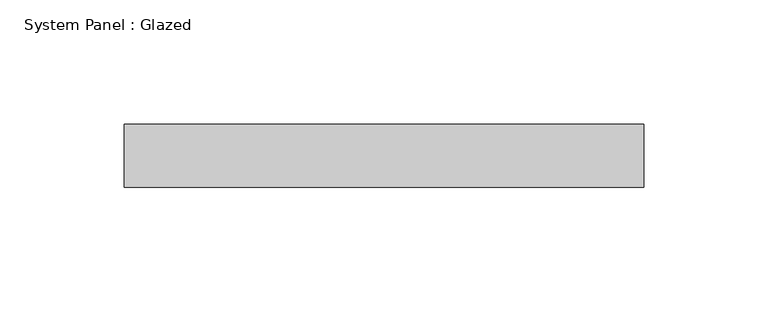
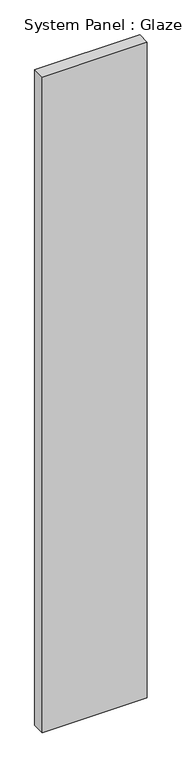
"""IFC4 building model written with IfcOpenShell, lengths in millimetres: plate geometry, System Panel : Glazed."""

from ifc_helpers import new_model, si_unit, origin, origin_with_axes, place, context, project, spatial, polyline, outline, extrude, source, transform, mapped, element, save


def system_panel_glazed_475412f8(model_context):
    return source(origin(), model_context, "Body", "SweptSolid", [
        extrude(outline(polyline([(104.775, 19.05), (-104.775, 19.05), (-104.775, 44.45), (104.775, 44.45), (104.775, 19.05)])), origin_with_axes(), (0.0, 0.0, 1.0), 1382.6020555),
    ])


if __name__ == "__main__":
    model = new_model("IFC4")
    model_context = context("Model", 3, world=origin())
    ifc_project = project(units=[si_unit("LENGTHUNIT", "METRE", prefix="MILLI")], contexts=[model_context])
    site = spatial("IfcSite", under=ifc_project)
    building = spatial("IfcBuilding", under=site)
    placement = place(None, origin())
    system_panel_glazed_shape = system_panel_glazed_475412f8(model_context)
    element("IfcPlate", 1, ObjectType="System Panel : Glazed", at=placement, inside=building, context=model_context, shape_type="MappedRepresentation", body=[
        mapped(system_panel_glazed_shape, transform((0.0, 0.0, 0.0), x_axis=(1.0, 0.0, 0.0), y_axis=(0.0, 1.0, 0.0), z_axis=(0.0, 0.0, 1.0))),
    ])
    save(model, "model.ifc")

# Revit data of these elements
# Type "System Panel : Glazed"
#   Construction Type Id = "GSP4R"
#   Analytic Construction = "1/8 in Pilkington single glazing"
#   Visual Light Transmittance = 0.9
#   Solar Heat Gain Coefficient = 0.86
#   Heat Transfer Coefficient (U) = 1.18115 BTU/(h·ft²·°F)
#   Define Thermal Properties by = 1
# Element 1 (IfcPlate, "System Panel : Glazed")
#   Materials on its faces: "Glass"
# Materials
#   "Glass": class "Glass", colour RGB 0 128 192, transparency 0.75, Description = "Soda Lime Glass", Cost = 0
